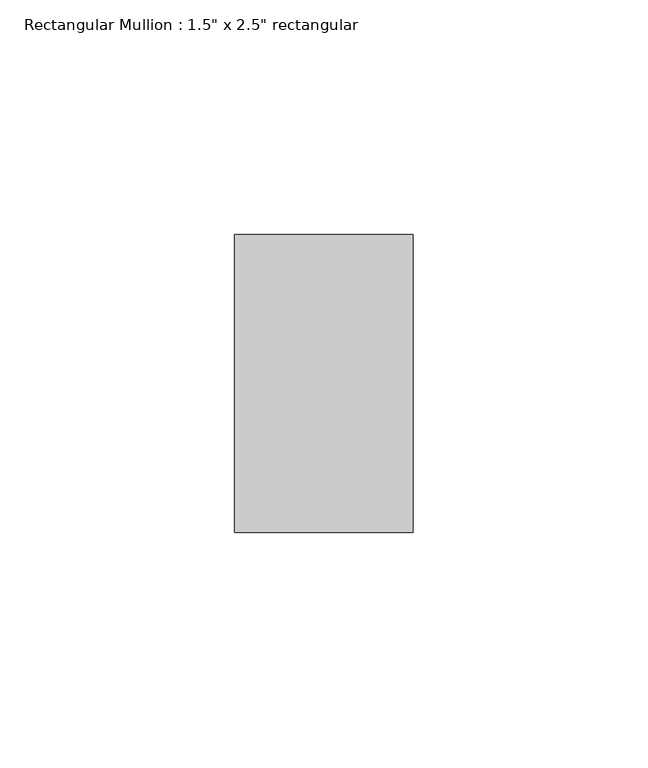
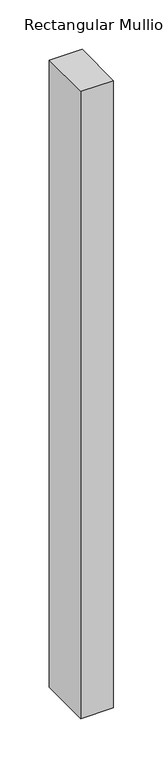
"""IFC4 building model written with IfcOpenShell, lengths in millimetres: member geometry."""

from ifc_helpers import new_model, si_unit, frame, origin, place, context, project, spatial, polyline, outline, extrude, source, transform, mapped, element, save


def member_55e892ad(model_context):
    return source(origin(), model_context, "Body", "SweptSolid", [
        extrude(outline(polyline([(19.05, 31.75), (19.05, -31.75), (-19.05, -31.75), (-19.05, 31.75), (19.05, 31.75)])), frame((0.0, 0.0, -774.7), z_axis=(0.0, 0.0, 1.0), x_axis=(1.0, 0.0, 0.0)), (0.0, 0.0, 1.0), 774.7),
    ])


if __name__ == "__main__":
    model = new_model("IFC4")
    model_context = context("Model", 3, world=origin())
    ifc_project = project(units=[si_unit("LENGTHUNIT", "METRE", prefix="MILLI")], contexts=[model_context])
    site = spatial("IfcSite", under=ifc_project)
    building = spatial("IfcBuilding", under=site)
    placement = place(None, origin())
    member_shape = member_55e892ad(model_context)
    element("IfcMember", 1, ObjectType="Rectangular Mullion : 1.5\" x 2.5\" rectangular", at=placement, inside=building, context=model_context, shape_type="MappedRepresentation", body=[
        mapped(member_shape, transform((0.0, 0.0, 0.0), x_axis=(1.0, 0.0, 0.0), y_axis=(0.0, 1.0, 0.0), z_axis=(0.0, 0.0, 1.0))),
    ])
    save(model, "model.ifc")

# Revit data of these elements
# Type "Rectangular Mullion : 1.5\" x 2.5\" rectangular"
#   built-in parameter 1007304 = 0.208333 (stored number, unit not read)
#   built-in parameter 1007301 = 0.0625 (stored number, unit not read)
#   built-in parameter 1007300 = 0.0625 (stored number, unit not read)
# Element 1 (IfcMember, "Rectangular Mullion : 1.5\" x 2.5\" rectangular")
#   Materials on its faces: "Leather - Black"
# Materials
#   "Leather - Black": class "Generic", colour RGB 40 40 40, transparency 0, Cost = 0
